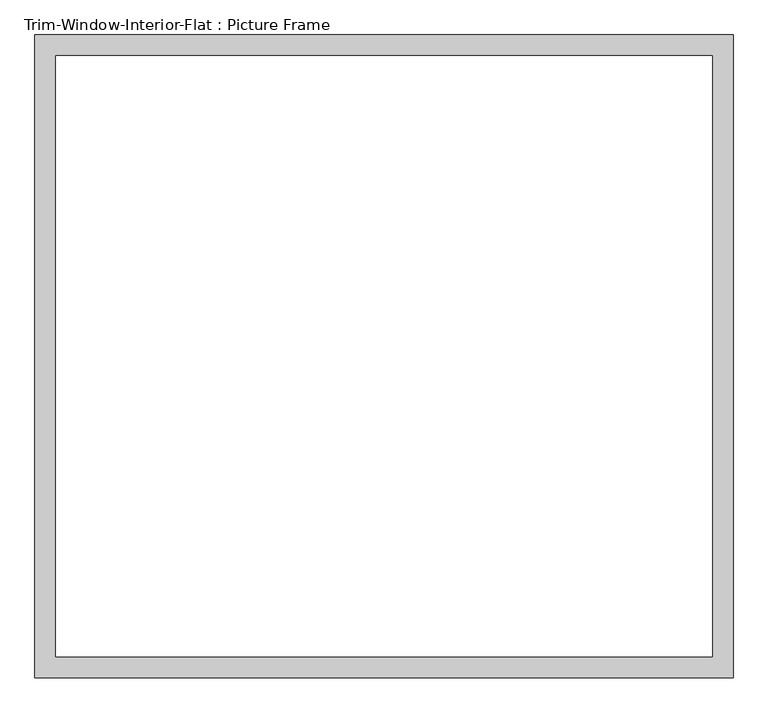
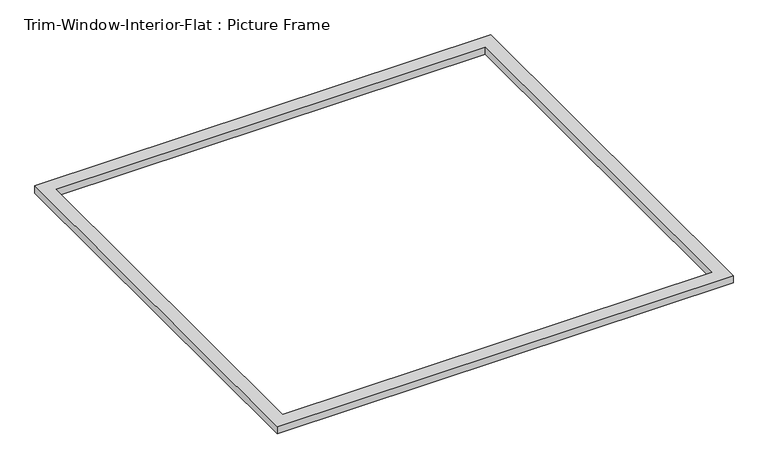
"""IFC4 building model written with IfcOpenShell, lengths in millimetres: proxy geometry, Trim-Window-Interior-Flat : Picture Frame."""

from ifc_helpers import new_model, si_unit, origin, origin_with_axes, place, context, project, spatial, polyline, outline, extrude, source, transform, mapped, element, save


def trim_window_interior_flat_picture_frame_b05ee221(model_context):
    return source(origin(), model_context, "Body", "SweptSolid", [
        extrude(outline(polyline([(958.85, 44.45), (958.85, -1720.85), (-958.85, -1720.85), (-958.85, 44.45), (958.85, 44.45)]), holes=[polyline([(901.7, -12.7), (-901.7, -12.7), (-901.7, -1663.7), (901.7, -1663.7), (901.7, -12.7)])]), origin_with_axes(), (0.0, 0.0, 1.0), 31.75),
    ])


if __name__ == "__main__":
    model = new_model("IFC4")
    model_context = context("Model", 3, world=origin())
    ifc_project = project(units=[si_unit("LENGTHUNIT", "METRE", prefix="MILLI")], contexts=[model_context])
    site = spatial("IfcSite", under=ifc_project)
    building = spatial("IfcBuilding", under=site)
    placement = place(None, origin())
    trim_window_interior_flat_picture_frame_shape = trim_window_interior_flat_picture_frame_b05ee221(model_context)
    element("IfcBuildingElementProxy", 1, Name="Trim-Window-Interior-Flat : Picture Frame", ObjectType="Trim-Window-Interior-Flat : Picture Frame", at=placement, inside=building, context=model_context, shape_type="MappedRepresentation", body=[
        mapped(trim_window_interior_flat_picture_frame_shape, transform((0.0, 0.0, 0.0), x_axis=(1.0, 0.0, 0.0), y_axis=(0.0, 1.0, 0.0), z_axis=(0.0, 0.0, 1.0))),
    ])
    save(model, "model.ifc")

# Revit data of these elements
# Type "Trim-Window-Interior-Flat : Picture Frame"
#   Trim Thickness_Picture Frame = 0' - 1 1/4"
#   Trim Width = 0' - 2 1/4"
#   Trim Thickness_with Sill = 0' - 0 3/4"
#   Sill Thickness = 0' - 1 1/4"
#   Opening Width [instance default] = 2' - 0"
#   Opening Height [instance default] = 3' - 0"
#   Default Elevation = 4' - 0"
#   Sill = no
#   Picture Frame = yes
#   Trim Material [instance default] = none
# Element 1 (IfcBuildingElementProxy, "Trim-Window-Interior-Flat : Picture Frame")
#   Opening Width = 6' - 0"
#   Opening Height = 5' - 6"
#   Trim Material = Wood - Stained
#   Materials on its faces: "Wood - Stained"
# Materials
#   "Wood - Stained": class "Wood", colour RGB 224 178 126, transparency 0, Cost = 0
